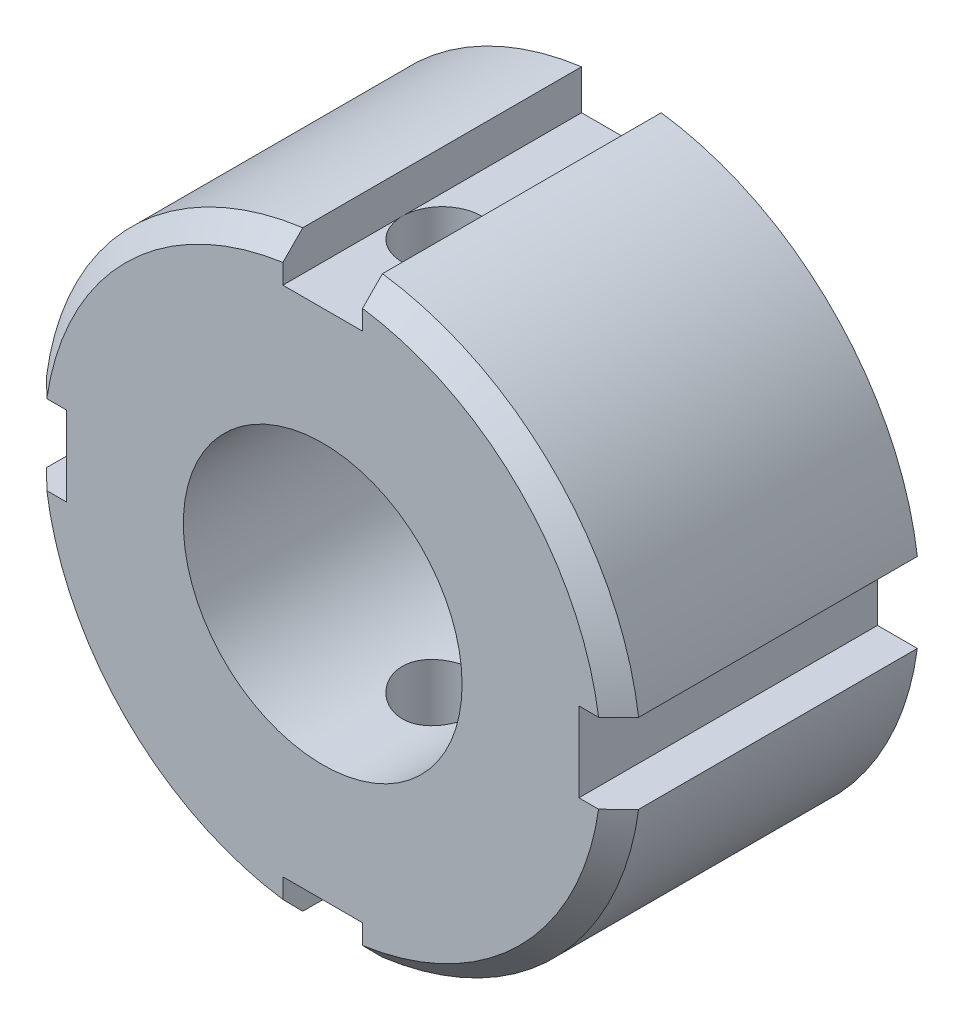
from build123d import *

# Parameters (mm, degrees)
NUT_BODY_15MM_DEPTH       = 7.5
M16_TAPPED_THROUGH_HOLE_D = 14
EDGE_CHAMFER_1X45_SIZE    = 1
CROSS_HOLE_4_DEPTH        = 23.321514286
CROSS_HOLE_4_DEPTH_BACK   = 23.321514286
CROSS_HOLE_4_SKETCH_R     = 2


with BuildPart() as part:
    # Slotted Nut Profile Ø30 → Nut Body 15mm (new, symmetric)
    with BuildSketch(Plane.XY):
        with BuildLine():
            Line((2, 12.866068747), (2, 14.866068747))
            ThreePointArc((2, 14.866068747), (10.606601718, 10.606601718), (14.866068747, 2))
            Line((14.866068747, 2), (12.866068747, 2))
            Line((12.866068747, 2), (12.866068747, -2))
            Line((12.866068747, -2), (14.866068747, -2))
            ThreePointArc((14.866068747, -2), (10.606601718, -10.606601718), (2, -14.866068747))
            Line((2, -14.866068747), (2, -12.866068747))
            Line((2, -12.866068747), (-2, -12.866068747))
            Line((-2, -12.866068747), (-2, -14.866068747))
            ThreePointArc((-2, -14.866068747), (-10.606601718, -10.606601718), (-14.866068747, -2))
            Line((-14.866068747, -2), (-12.866068747, -2))
            Line((-12.866068747, -2), (-12.866068747, 2))
            Line((-12.866068747, 2), (-14.866068747, 2))
            ThreePointArc((-14.866068747, 2), (-10.606601718, 10.606601718), (-2, 14.866068747))
            Line((-2, 14.866068747), (-2, 12.866068747))
            Line((-2, 12.866068747), (2, 12.866068747))
        make_face()
    extrude(amount=NUT_BODY_15MM_DEPTH, both=True)

    # M16 Tapped Through Hole (through all)
    with Locations(Plane.XY.offset(7.5)):
        with Locations((0, 0)):
            Hole(M16_TAPPED_THROUGH_HOLE_D / 2)

    # Edge Chamfer 1x45°
    edge_chamfer_1x45_edges = [part.edges().sort_by_distance(p)[0] for p in [
        (-10.606601718, 10.606601718, 7.5),
        (-10.606601718, -10.606601718, 7.5),
        (10.606601718, -10.606601718, 7.5),
        (10.606601718, 10.606601718, 7.5),
    ]]
    chamfer(edge_chamfer_1x45_edges, length=EDGE_CHAMFER_1X45_SIZE)

    # Cross Hole Ø4 Sketch → Cross Hole Ø4 (cut, two sides: drawn at the far end of the back side and taken through both)
    with BuildSketch(Plane(origin=(0, 0, 0), x_dir=(1, 0, 0), z_dir=(0, 1, 0)).offset(-CROSS_HOLE_4_DEPTH_BACK)):
        with Locations(Location((0, -1.5, 0), (0, 0, 270))):
            Circle(CROSS_HOLE_4_SKETCH_R)
    extrude(amount=CROSS_HOLE_4_DEPTH + CROSS_HOLE_4_DEPTH_BACK, mode=Mode.SUBTRACT)


solid = part.part
